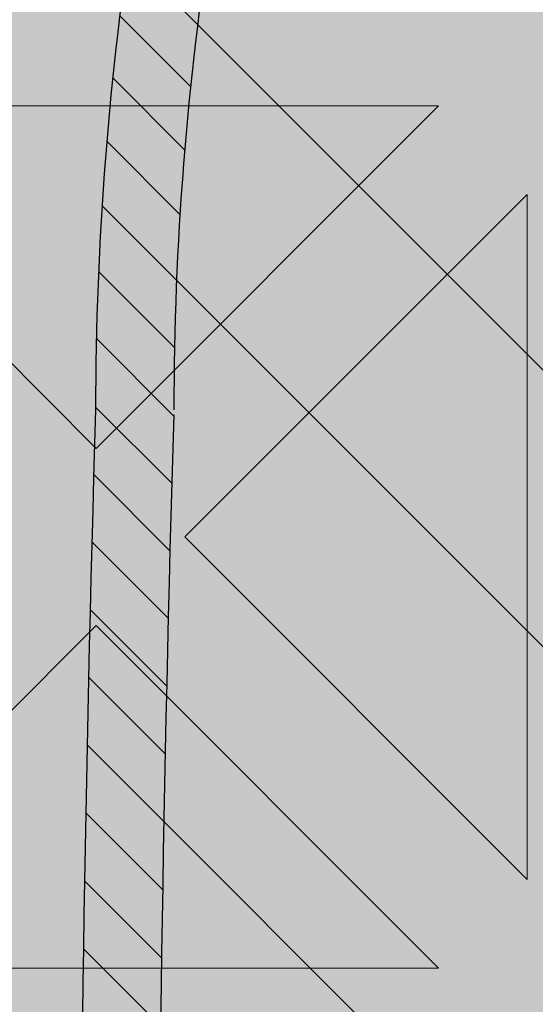
# Model space of a CAD drawing. Units: inches. Extents: x 844 to 2234, y 346 to 1084.
# Tile 78 of 93: x 2000.116 to 2001.166, y 704.51 to 706.514. Entities that reach past the tile are written whole.
import ezdxf

# ---------------------------------------------------------------- set-up
doc = ezdxf.new("R2010")
doc.units = ezdxf.units.IN
doc.header["$MEASUREMENT"] = 0
for name, color, linetype, lineweight in [('A-ANNO-DIMS', 2, 'Continuous', 18), ('furniture', 8, 'Continuous', 18), ('RA-AP-01$0$INT', 35, 'Continuous', 5)]:
    doc.layers.add(name, color=color, linetype=linetype, lineweight=lineweight)
doc.layers.add('RA-AP-01$0$FURN', color=3, linetype='Continuous')
doc.layers.add('RA-AP-01$0$WOOD', color=64, linetype='Continuous')
doc.styles.get("Standard").update_dxf_attribs({"font": 'arial.ttf'})
doc.dimstyles.get("Standard").update_dxf_attribs({"dimtxt": 6, "dimasz": 3, "dimexe": 0.18, "dimexo": 0.0625, "dimgap": 0.09, "dimtad": 0, "dimtih": 1, "dimtoh": 1, "dimdec": 1, "dimzin": 0, "dimdsep": 46, "dimlunit": 3, "dimtxsty": 'Standard', "dimblk": 'ARCHTICK', "dimcen": 0.09, "dimadec": 0, "dimazin": 0, "dimtfac": 1, "dimtdec": 1, "dimtofl": 0, "dimtmove": 0, "dimatfit": 3, "dimfxl": 1, "dimtolj": 1, "dimtzin": 0, "dimarcsym": 0})

# ---------------------------------------------------------------- blocks, each defined once
blk = doc.blocks.new('A$C18D01794')
at = {"layer": 'RA-AP-01$0$INT'}
h = blk.add_hatch(color=256, dxfattribs=at)
h.paths.add_polyline_path([(4.585917135068448, -7.856712009587804), (4.614201406330596, -7.856712009587056), (4.668846067270487, -7.802067348644738), (4.723490728212344, -7.856712009584164), (4.771774999457151, -7.856712009582887), (4.826419660396886, -7.80206734864072), (4.862780050090322, -7.838427738332541), (4.844495778842715, -7.856712009580965), (4.862780050090411, -7.856712009580482), (4.905206456960182, -7.814285602707865), (4.947632863832445, -7.856712009578238), (4.965917135079675, -7.856712009577755), (4.947632863831759, -7.838427738330656), (4.983993253523576, -7.802067348637219), (5.038637914464627, -7.856712009575829), (5.08692218571208, -7.856712009574554), (5.141566846649976, -7.802067348634224), (5.196211507589851, -7.856712009571666), (5.224495778822615, -7.856712009570916), (4.905206456953975, -7.537422687702283)])
h.paths.add_polyline_path([(4.895206456956031, -7.575706958950402), (4.895206456958921, -7.684996280828174), (4.840561796018589, -7.630351619890275)], flags=16)
h.paths.add_polyline_path([(4.915206456955638, -7.575706958949956), (4.969851117895509, -7.630351619887399), (4.915206456957609, -7.684996280827732)], flags=16)
h.paths.add_polyline_path([(4.826419660395175, -7.644493755514321), (4.881064321335613, -7.699138416452331), (4.771774999456703, -7.69913841645522)], flags=16)
h.paths.add_polyline_path([(4.983993253519558, -7.644493755510815), (5.038637914460456, -7.699138416449285), (4.929348592581548, -7.69913841645126)], flags=16)
h.paths.add_polyline_path([(4.881064321336025, -7.719138416452334), (4.826419660397532, -7.773783077393256), (4.771774999457062, -7.719138416455217)], flags=16)
h.paths.add_polyline_path([(4.929348592582019, -7.71913841645126), (5.038637914460982, -7.719138416449284), (4.983993253522945, -7.773783077389749)], flags=16)
h.paths.add_polyline_path([(4.895206456960191, -7.733280552075633), (4.895206456962115, -7.806001331460164), (4.876922185715016, -7.824285602708492), (4.840561796021581, -7.787925213016675)], flags=16)
h.paths.add_polyline_path([(4.915206456958487, -7.733280552075187), (4.969851117899527, -7.787925213013798), (4.933490728206909, -7.824285602708034), (4.9152064569598, -7.806001331461736)], flags=16)
h.paths.add_polyline_path([(4.757632863832376, -7.733280552079264), (4.812277524772842, -7.787925213017304), (4.757632863834348, -7.842569873958233)], flags=16)
h.paths.add_polyline_path([(4.737632863832376, -7.73328055207979), (4.737632863834348, -7.842569873958701), (4.682988202893906, -7.787925213020692)], flags=16)
h.paths.add_polyline_path([(5.05278005008503, -7.733280552072701), (5.052780050087917, -7.842569873951664), (4.998135389146995, -7.787925213013169)], flags=16)
h.paths.add_polyline_path([(5.072780050085024, -7.733280552072333), (5.127424711025931, -7.787925213010806), (5.072780050087916, -7.842569873951244)], flags=16)
h.paths.add_polyline_path([(4.935917135072783, -7.506712009583784), (5.255206456948811, -7.826001331459767), (5.255206456948932, -7.797717060211899), (5.200561796010279, -7.743072399273238), (5.255206456949403, -7.688427738334128), (5.25520645694961, -7.640143467086677), (5.200561796009787, -7.585498806146837), (5.236922185702417, -7.549138416454212), (5.255206456949919, -7.56742268770172), (5.255206456949998, -7.549138416454178), (5.212780050078687, -7.506712009583814), (5.25520645695036, -7.464285602712145), (5.255206456950438, -7.446001331464763), (5.236922185702424, -7.464285602712779), (5.200561796009796, -7.427925213020149), (5.255206456950753, -7.373280552079203), (5.25520645695096, -7.324996280834394), (5.200561796010322, -7.270351619893748), (5.255206456951428, -7.215706958952649), (5.255206456951547, -7.187422687705071)])
h.paths.add_polyline_path([(5.042988202883395, -7.42792521302065), (5.097632863823085, -7.373280552080975), (5.097632863822622, -7.482569873959883)], flags=16)
h.paths.add_polyline_path([(5.028846067259663, -7.442067348644384), (5.083490728198774, -7.496712009583504), (4.974201406321001, -7.496712009583035)], flags=16)
h.paths.add_polyline_path([(5.117632863823087, -7.37328055208089), (5.172277524762331, -7.42792521302015), (5.11763286382262, -7.482569873959851)], flags=16)
h.paths.add_polyline_path([(5.08349072819877, -7.516712009582191), (5.028846067259652, -7.571356670521302), (4.974201406320998, -7.516712009582638)], flags=16)
h.paths.add_polyline_path([(5.131774999446817, -7.35913841645716), (5.186419660386065, -7.413783077396415), (5.241064321325782, -7.359138416456712)], flags=17)
h.paths.add_polyline_path([(5.131774999446228, -7.496712009583703), (5.186419660386065, -7.442067348643883), (5.222780050079488, -7.478427738337313), (5.204495778832781, -7.496712009584014)], flags=16)
h.paths.add_polyline_path([(5.097632863822613, -7.530854145205813), (5.097632863823061, -7.640143467084723), (5.042988202883383, -7.585498806145032)], flags=16)
h.paths.add_polyline_path([(5.131774999446899, -7.339138416457162), (5.241064321325809, -7.339138416456712), (5.186419660386591, -7.284493755517479)], flags=17)
h.paths.add_polyline_path([(5.131774999446226, -7.516712009581999), (5.204495778830767, -7.516712009581702), (5.22278005007868, -7.534996280829206), (5.186419660386049, -7.571356670521828)], flags=16)
h.paths.add_polyline_path([(5.11763286382262, -7.530854145205852), (5.17227752476232, -7.585498806145562), (5.117632863823064, -7.64014346708481)], flags=16)
h.paths.add_polyline_path([(5.186419660386069, -7.599640941770585), (5.241064321325754, -7.654285602710281), (5.131774999446791, -7.654285602709814)], flags=16)
h.paths.add_polyline_path([(5.131774999446872, -7.674285602709813), (5.24106432132578, -7.674285602710282), (5.186419660386554, -7.728930263649504)], flags=16)
h.paths.add_polyline_path([(5.255206456951811, -7.126001331467467), (5.255206456951895, -7.106712009588038), (4.555206456956052, -7.106712009588038), (4.555206456956136, -7.12600133146746), (4.905206456953973, -7.476001331465289)])
h.paths.add_polyline_path([(4.983993253513404, -7.368930263651977), (4.92934859257295, -7.314285602713969), (5.03863791445186, -7.314285602711063)], flags=16)
h.paths.add_polyline_path([(4.969851117889988, -7.383072399276016), (4.915206456952556, -7.437717060215906), (4.915206456949648, -7.328427738338133)], flags=16)
h.paths.add_polyline_path([(4.929348592572535, -7.294285602713971), (4.983993253511019, -7.239640941773039), (5.038637914451496, -7.294285602711065)], flags=16)
h.paths.add_polyline_path([(5.052780050074912, -7.280143467087016), (4.998135389134438, -7.225498806148989), (5.052780050072919, -7.170854145208052)], flags=16)
h.paths.add_polyline_path([(5.07278005007491, -7.280143467086489), (5.072780050072918, -7.170854145207579), (5.127424711013374, -7.225498806145578)], flags=16)
h.paths.add_polyline_path([(4.89520645695295, -7.437717060216355), (4.840561796013067, -7.383072399278919), (4.895206456950961, -7.328427738338582)], flags=16)
h.paths.add_polyline_path([(4.915206456948365, -7.280143467090674), (4.915206456946434, -7.207422687704125), (4.933490728192729, -7.18913841645701), (4.969851117886972, -7.225498806149623)], flags=16)
h.paths.add_polyline_path([(4.881064321327021, -7.314285602715054), (4.82641966038902, -7.368930263655506), (4.771774999448108, -7.314285602717047)], flags=16)
h.paths.add_polyline_path([(4.895206456950073, -7.280143467091125), (4.840561796009022, -7.225498806152518), (4.876922185700835, -7.18913841645908), (4.895206456948749, -7.207422687706589)], flags=16)
h.paths.add_polyline_path([(4.983993253510392, -7.211356670525576), (4.947632863816944, -7.174996280833758), (4.965917135064043, -7.156712009585847), (5.038637914448995, -7.156712009584522)], flags=16)
h.paths.add_polyline_path([(4.881064321326543, -7.294285602715056), (4.771774999447578, -7.294285602717046), (4.826419660385607, -7.239640941776569)], flags=16)
h.paths.add_polyline_path([(4.905206456946447, -7.19913841645844), (4.862780050074785, -7.156712009587725), (4.947632863816685, -7.156712009586302)], flags=16)
h.paths.add_polyline_path([(5.14156684663679, -7.211356670521528), (5.086922185696452, -7.156712009583639), (5.196211507574223, -7.156712009581651)], flags=16)
h.paths.add_polyline_path([(4.8264196603837, -7.211356670529104), (4.771774999442643, -7.156712009590501), (4.8444957788276, -7.156712009588568), (4.862780050075511, -7.17499628083566)], flags=16)
h.paths.add_polyline_path([(4.812277524760289, -7.225498806153156), (4.757632863822258, -7.28014346709363), (4.757632863819352, -7.170854145214669)], flags=16)
h.paths.add_polyline_path([(4.73763286382226, -7.280143467093997), (4.682988202881349, -7.22549880615554), (4.737632863819352, -7.170854145215086)], flags=16)
h.paths.add_polyline_path([(4.723490728195188, -7.156712009591787), (4.668846067257299, -7.211356670532127), (4.614201406317417, -7.156712009594693)], flags=16)
h.paths.add_polyline_path([(4.597632863829262, -7.506712009583814), (4.555206456957951, -7.54913841645418), (4.555206456958029, -7.56742268770172), (4.573490728205535, -7.549138416454212), (4.609851117898167, -7.585498806146839), (4.555206456958338, -7.640143467086675), (4.555206456958546, -7.688427738334125), (4.60985111789767, -7.743072399273238), (4.555206456959015, -7.797717060211899), (4.555206456959138, -7.826001331459767), (4.874495778835167, -7.506712009583786), (4.5552064569564, -7.187422687705062), (4.555206456956523, -7.215706958952644), (4.609851117897629, -7.270351619893746), (4.555206456956988, -7.324996280834396), (4.555206456957198, -7.373280552079195), (4.609851117898153, -7.427925213020147), (4.573490728205528, -7.464285602712779), (4.555206456957507, -7.446001331464756), (4.555206456957585, -7.464285602712143)])
h.paths.add_polyline_path([(4.712780050085332, -7.482569873959882), (4.712780050084863, -7.373280552080972), (4.767424711024555, -7.42792521302065)], flags=16)
h.paths.add_polyline_path([(4.726922185709173, -7.496712009583504), (4.781566846648288, -7.442067348644384), (4.836211507586949, -7.496712009583033)], flags=16)
h.paths.add_polyline_path([(4.692780050085327, -7.482569873959851), (4.638135389145619, -7.427925213020149), (4.692780050084865, -7.373280552080892)], flags=16)
h.paths.add_polyline_path([(4.726922185709182, -7.516712009582191), (4.836211507586949, -7.51671200958264), (4.7815668466483, -7.571356670521304)], flags=16)
h.paths.add_polyline_path([(4.678637914461726, -7.496712009583706), (4.605917135075169, -7.496712009584014), (4.587632863828464, -7.478427738337311), (4.623993253521887, -7.442067348643881)], flags=16)
h.paths.add_polyline_path([(4.712780050085336, -7.530854145205816), (4.767424711024568, -7.585498806145034), (4.71278005008489, -7.640143467084724)], flags=16)
h.paths.add_polyline_path([(4.678637914461726, -7.516712009582001), (4.623993253521899, -7.571356670521829), (4.587632863829271, -7.534996280829206), (4.605917135077185, -7.5167120095817)], flags=16)
h.paths.add_polyline_path([(4.692780050085336, -7.530854145205848), (4.692780050084889, -7.64014346708481), (4.638135389145632, -7.585498806145562)], flags=16)
h.paths.add_polyline_path([(4.623993253521885, -7.413783077396415), (4.678637914461131, -7.359138416457161), (4.56934859258217, -7.359138416456712)], flags=17)
h.paths.add_polyline_path([(4.623993253521901, -7.599640941770568), (4.678637914461158, -7.654285602709814), (4.569348592582195, -7.654285602710281)], flags=16)
h.paths.add_polyline_path([(4.678637914461051, -7.339138416457162), (4.623993253521361, -7.284493755517479), (4.569348592582143, -7.339138416456712)], flags=17)
h.paths.add_polyline_path([(4.678637914461076, -7.674285602709813), (4.623993253521399, -7.728930263649504), (4.569348592582167, -7.674285602710281)], flags=16)
h = blk.add_hatch(color=256, dxfattribs=at)
h.paths.add_polyline_path([(5.028846067259997, -7.571356670520955), (4.974201406321342, -7.516712009582294), (5.083490728199115, -7.516712009581846)])
h.paths.add_polyline_path([(4.974201406321344, -7.496712009582688), (5.028846067260004, -7.442067348644037), (5.083490728199117, -7.496712009583157)])
h.paths.add_polyline_path([(5.042988202883738, -7.427925213020309), (5.097632863823428, -7.373280552080627), (5.097632863822963, -7.482569873959537)])
h.paths.add_polyline_path([(5.117632863822961, -7.482569873959509), (5.117632863823428, -7.373280552080546), (5.172277524762674, -7.427925213019804)])
h.paths.add_polyline_path([(5.131774999446572, -7.496712009583358), (5.186419660386406, -7.442067348643536), (5.222780050079831, -7.478427738336961), (5.204495778833122, -7.496712009583667)])
h.paths.add_polyline_path([(5.236922185702764, -7.464285602712433), (5.200561796010139, -7.427925213019802), (5.255206456949971, -7.373280552079975), (5.255206456950271, -7.446001331464927)])
h.paths.add_polyline_path([(5.186419660386412, -7.41378307739607), (5.131774999447164, -7.359138416456815), (5.241064321326123, -7.359138416456366)])
h.paths.add_polyline_path([(5.131774999447238, -7.339138416456815), (5.186419660386934, -7.284493755517132), (5.241064321326153, -7.339138416456368)])
h.paths.add_polyline_path([(5.200561796010663, -7.270351619893402), (5.255206456949324, -7.215706958954747), (5.255206456949777, -7.324996280832518)])
h.paths.add_polyline_path([(5.21278005007903, -7.50671200958347), (5.255206456950223, -7.464285602712278), (5.255206456950696, -7.549138416454185)])
h.paths.add_polyline_path([(5.13177499944657, -7.516712009581652), (5.204495778831106, -7.516712009581354), (5.222780050079024, -7.534996280828858), (5.186419660386397, -7.571356670521485)])
h.paths.add_polyline_path([(5.117632863823405, -7.640143467084465), (5.117632863822955, -7.530854145205498), (5.172277524762665, -7.585498806145217)])
h.paths.add_polyline_path([(5.042988202883727, -7.585498806144689), (5.097632863822957, -7.530854145205474), (5.097632863823407, -7.64014346708438)])
h.paths.add_polyline_path([(5.131774999447135, -7.654285602709467), (5.186419660386394, -7.599640941770219), (5.241064321326097, -7.654285602709933)])
h.paths.add_polyline_path([(5.200561796010128, -7.585498806146492), (5.236922185702758, -7.549138416453866), (5.255206456950264, -7.567422687701371), (5.255206456949948, -7.640143467086325)])
h.paths.add_polyline_path([(5.186419660386895, -7.728930263649157), (5.131774999447213, -7.674285602709467), (5.241064321326127, -7.674285602709934)])
h.paths.add_polyline_path([(5.200561796010624, -7.743072399272893), (5.255206456949745, -7.688427738333778), (5.255206456949276, -7.797717060211553)])
for p, q in [((5.131774999446817, -7.359138416457161), (5.24106432132578, -7.359138416456712)), ((5.131774999446817, -7.359138416457161), (5.186419660386065, -7.413783077396415)), ((5.24106432132578, -7.359138416456712), (5.186419660386065, -7.413783077396415)), ((5.117632863823085, -7.37328055208089), (5.172277524762331, -7.427925213020149)), ((5.117632863823085, -7.37328055208089), (5.11763286382262, -7.482569873959853)), ((5.11763286382262, -7.482569873959853), (5.172277524762331, -7.427925213020149)), ((5.131774999446229, -7.496712009583704), (5.186419660386063, -7.442067348643881)), ((5.186419660386062, -7.442067348643881), (5.222780050078687, -7.478427738336511)), ((5.204495778831181, -7.496712009584014), (5.131774999446229, -7.496712009583704))]:
    blk.add_line(p, q, dxfattribs=at)
blk = doc.blocks.new('A$C32926AE1')
at = {"layer": 'RA-AP-01$0$WOOD'}
h = blk.add_hatch(color=256, dxfattribs=at)
h.dxf.hatch_style = 1
h.paths.add_polyline_path([(5.157430609644524, 4.573483066760929, -0.1009492694046607), (5.155401577623758, 4.593365984175333, -0.1842662638101597), (5.172249623284174, 4.638795604568598, 0.2056608120311276), (5.179560981299304, 4.661316324430096, 0.3614336704623542), (5.134352340494423, 4.706524965234944, 0.2056608120311297), (5.111831620632933, 4.699213607219793, -0.1842662638101113), (5.066402000239693, 4.682365561559342, -0.1055311479399994), (5.045656153913092, 4.68467289944697, 0.1567636581983829), (4.763886414745334, 4.684672899446966, -0.1055311479399895), (4.743140568418733, 4.68236556155934, -0.1842662638100833), (4.6977109480255, 4.69921360721979, 0.2056608120302612), (4.675190228164109, 4.706524965234949, 0.3614336704708441), (4.629981587358889, 4.66131632442871, 0.2056608120245944), (4.637292945374126, 4.638795604567974, -0.1842662638101024), (4.654140991034615, 4.59336598417475, -0.1009492694055169), (4.652111959013835, 4.573483066760181, 0.021410119221476), (4.629748025606143, 4.156712009541676, 0.0214101192214795), (4.652111959013809, 3.739940952323101, -0.1009492694059586), (4.654140991034615, 3.720058034908448, -0.1842662638100975), (4.637292945374126, 3.674628414515226, 0.2056608120245705), (4.629981587358889, 3.652107694654492, 0.3614336704708879), (4.675190228164113, 3.606899053848249, 0.2056608120302384), (4.697710948025501, 3.614210411863408, -0.1842662638100995), (4.743140568418738, 3.63105845752386, -0.1055311479402541), (4.763886414745388, 3.628751119636215, 0.1567636581983776), (5.045656153913137, 3.628751119636244, -0.1055311479397538), (5.066402000239692, 3.631058457523857, -0.1842662638101067), (5.111831620632931, 3.614210411863407, 0.2056608120310924), (5.134352340494417, 3.606899053848256, 0.3614336704624001), (5.179560981299307, 3.652107694653103, 0.2056608120311314), (5.172249623284175, 3.6746284145146, -0.1842662638101402), (5.155401577623758, 3.72005803490786, -0.1009492694051366), (5.15743060964455, 3.739940952322354, 0.0214101192215073), (5.179794543052287, 4.156712009541468, 0.0214101192215252)])
h.paths.add_polyline_path([(4.639748609479751, 4.156712009541513, 0.0213537860821624), (4.661970494867118, 3.741887061152232, -0.094075836301374), (4.664143710413708, 3.7196126951003, -0.1824818158568985), (4.644813765429836, 3.668037719127816, 0.2056608120245319), (4.639939526753007, 3.653023905887301, 0.3614336704710246), (4.676106439397173, 3.616856993242342, 0.2056608120302234), (4.691120252638095, 3.621731231919122, -0.1824818158602558), (4.742695228611606, 3.641061176902986, -0.1029891339458722), (4.766991894714349, 3.638256818950944, 0.156709409989566), (5.042550673941472, 3.638256818950105, -0.102989133958497), (5.066847340047078, 3.641061176902949, -0.1824818158594995), (5.118422316020358, 3.621731231919103, 0.2056608120311416), (5.133436129261316, 3.616856993242346, 0.3614336704621468), (5.169603041905217, 3.653023905886178, 0.2056608120310986), (5.164728803228477, 3.668037719127177, -0.1824818158565612), (5.145398858244737, 3.719612695099578, -0.0940758363009313), (5.147572073791232, 3.741887061151398, 0.0213537860822023), (5.169793959178681, 4.156712009541451, 0.0213537860822226), (5.147572073791203, 4.571536957931898, -0.0940758363005034), (5.145398858244737, 4.59381132398362, -0.1824818158565587), (5.164728803228476, 4.645386299956021, 0.2056608120311045), (5.169603041905216, 4.66040011319702, 0.3614336704621845), (5.133436129261313, 4.696567025840856, 0.2056608120310773), (5.118422316020359, 4.691692787164098, -0.182481815859508), (5.066847340047078, 4.67236284218025, -0.1029891339584606), (5.04255067394148, 4.675167200133092, 0.156709409989566), (4.766991894714357, 4.675167200132257, -0.1029891339458842), (4.742695228611611, 4.672362842180213, -0.1824818158602725), (4.691120252638095, 4.691692787164077, 0.2056608120302152), (4.676106439397174, 4.696567025840858, 0.3614336704710363), (4.639939526753005, 4.660400113195899, 0.2056608120245495), (4.644813765429837, 4.645386299955384, -0.1824818158568934), (4.664143710413708, 4.593811323982902, -0.0940758363009187), (4.661970494867149, 4.571536957931074, 0.021353786082177)], flags=16)
h.paths.add_polyline_path([(5.129794543052235, 4.432167055276933, -0.0141661062790638), (5.130152669293814, 4.156927903047693, -0.0141661062790647), (5.129794543052234, 3.881688750818433, -0.0785247771143638), (5.10979738006795, 3.755143611847103, 0.0945969212073497), (5.105408519571111, 3.717898134952927, 0.1043170707844957), (5.116074640131521, 3.670385395016088, 0.1043170707864965), (5.068561900193738, 3.681051515576561, 0.09459692119553), (5.031316423304057, 3.676662655080835, -0.1580239521427272), (4.778226145355827, 3.676662655080367, 0.0945969211986668), (4.740980668464973, 3.681051515576592, 0.1043170707882822), (4.693467928526415, 3.670385395015844, 0.1043170707867916), (4.704134049087309, 3.717898134953662, 0.0945969211972894), (4.69974518859162, 3.755143611844042, -0.0785247771163196), (4.679748025606343, 3.881688750818406, -0.0141661062790663), (4.679389899364763, 4.156927903047693, -0.0141661062790672), (4.679748025606343, 4.432167055276998, -0.0785247771163064), (4.699745188591625, 4.55871219425134, 0.094596921197333), (4.704134049087308, 4.595957671141738, 0.1043170707867205), (4.693467928526416, 4.643470411079523, 0.1043170707882628), (4.740980668464965, 4.632804290518776, 0.0945969211988114), (4.778226145355874, 4.637193151015016, -0.158023952142669), (5.031316423304015, 4.637193151014546, 0.0945969211956361), (5.068561900193736, 4.632804290518806, 0.1043170707864979), (5.11607464013152, 4.643470411079278, 0.1043170707844617), (5.105408519571112, 4.595957671142455, 0.0945969212074597), (5.109797380067959, 4.558712194248236, -0.0785247771143467)], flags=0)
h.paths.add_polyline_path([(5.119794532311105, 4.432259799204851, -0.0142000800617244), (5.120156169157484, 4.156927903047701, -0.0142000800617277), (5.119794532311105, 3.881596006890482, -0.0784894509520253), (5.100273383573699, 3.758192358677797, 0.0940138827242913), (5.095413455884425, 3.717477693979438, 0.0606271852308753), (5.099615656341024, 3.686844378806616, 0.0606271852322524), (5.068982341167493, 3.691046579263239, 0.0940138827010453), (5.028267676478798, 3.686186651576848, -0.1580706864508061), (4.781274892180912, 3.686186651576435, 0.0940138827026903), (4.740560227491556, 3.691046579263279, 0.0606271852339895), (4.709926912317155, 3.686844378806508, 0.0606271852329405), (4.714129112773991, 3.717477693980356, 0.094013882701304), (4.709269185087677, 3.758192358669163, -0.0784894509577193), (4.689748036347473, 3.881596006890469, -0.014200080061729), (4.689386399501094, 4.156927903047709, -0.0142000800617217), (4.689748036347473, 4.432259799204808, -0.078489450957724), (4.709269185087651, 4.555663447426125, 0.0940138827014585), (4.714129112773992, 4.596378112114996, 0.0606271852329731), (4.709926912317154, 4.62701142728886, 0.0606271852340196), (4.74056022749157, 4.622809226832087, 0.0940138827024997), (4.781274892180847, 4.627669154518912, -0.1580706864508359), (5.028267676478777, 4.627669154518526, 0.0940138827010946), (5.068982341167492, 4.622809226832129, 0.060627185232254), (5.099615656341024, 4.627011427288751, 0.0606271852308727), (5.095413455884425, 4.59637811211593, 0.0940138827241088), (5.100273383573675, 4.555663447417647, -0.0784894509520978)], flags=0)
h.paths.add_polyline_path([(5.06978912287499, 4.430218106756144, -0.014241683694547), (5.070173729147532, 4.156927903047672, -0.0142416836945458), (5.06978912287499, 3.883637699339223, -0.0800609523125196), (5.052662118612511, 3.773463122773442, 0.0526421978001116), (5.04590916754064, 3.740550867606997, 0.0526421977992423), (5.012996912374707, 3.73379791653534, -0.1583028414718258), (4.796545656286308, 3.73379791653451, 0.0526421978034211), (4.763633401117837, 3.740550867607021, 0.0526421978018622), (4.756880450045755, 3.773463122774558, -0.0800609523117106), (4.739753445783639, 3.883637699339268, -0.0142416836945435), (4.739368839511098, 4.156927903047671, -0.0142416836945477), (4.739753445783639, 4.430218106756155, -0.0800609523116345), (4.75688045004574, 4.540392683320762, 0.052642197801941), (4.763633401117837, 4.573304938488346, 0.0526421978035071), (4.796545656286361, 4.580057889560873, -0.1583028414717561), (5.012996912374669, 4.580057889560039, 0.0526421977993048), (5.04590916754064, 4.57330493848837, 0.0526421978002057), (5.052662118612529, 4.540392683321868, -0.080060952312477)], flags=0)
h.paths.add_polyline_path([(5.049789715110557, 4.43038092723357, -0.0143097550741839), (5.05018085590259, 4.156927903047715, -0.0143097550741854), (5.049789715110558, 3.883474878861827, -0.0800685599149176), (5.03362098255317, 3.779581877367999, 0.0306258898956367), (5.028241146483733, 3.758218888663947, 0.0306258898977031), (5.006878157778253, 3.75283905259408, -0.1583983521624096), (4.802664410878162, 3.752839052594731, 0.0306258898946014), (4.781301422174808, 3.758218888663924, 0.0306258898967912), (4.775921586105202, 3.779581877368794, -0.080068559914251), (4.759752853548071, 3.883474878861786, -0.0143097550741854), (4.759361712756037, 4.156927903047671, -0.0143097550741854), (4.759752853548071, 4.430380927233557, -0.0800685599142479), (4.775921586105193, 4.534273928726546, 0.0306258898968306), (4.781301422174808, 4.555636917431444, 0.0306258898945754), (4.802664410878143, 4.561016753500631, -0.1583983521624168), (5.006878157778244, 4.561016753501291, 0.0306258898977177), (5.028241146483733, 4.555636917431421, 0.0306258898958182), (5.03362098255321, 4.534273928727244, -0.080068559914796)], flags=0)
h.paths.add_polyline_path([(4.999766070382627, 4.428171244713864, -0.0143443147609634), (5.000198441819402, 4.156927903047689, -0.0143443147609612), (4.999766070382627, 3.885684561381556, -0.0784641635803329), (4.987356730658798, 3.799103304488872, -0.1506053783831347), (4.822185837999821, 3.79910330448882, -0.0784641635803318), (4.809776498276007, 3.885684561381509, -0.014344314760963), (4.809344126839227, 4.156927903047677, -0.0143443147609645), (4.809776498276007, 4.428171244713873, -0.0784641635803192), (4.822185837999822, 4.514752501606549, -0.1506053783831338), (4.987356730658798, 4.514752501606494, -0.078464163580285)], flags=0)
h.paths.add_polyline_path([(4.979755254238824, 4.42764379880488, -0.0143772539198268), (4.980205517789977, 4.156927903047693, -0.0143772539198275), (4.979755254238824, 3.886212007290489, -0.0689242507424422), (4.971183264704897, 3.815276770442801, -0.1296645318904179), (4.838359303953726, 3.815276770442746, -0.0689242507424186), (4.829787314419809, 3.886212007290419, -0.0143772539198292), (4.829337050868653, 4.156927903047653, -0.0143772539198325), (4.829787314419809, 4.427643798804946, -0.0689242507424211), (4.838359303953725, 4.498579035652621, -0.1296645318904187), (4.971183264704897, 4.498579035652565, -0.0689242507424401)], flags=0)
h = blk.add_hatch(color=256, dxfattribs=at)
h.dxf.hatch_style = 1
h.paths.add_polyline_path([(5.145398858244737, 4.59381132398362, -0.1824818158565616), (5.164728803228476, 4.645386299956021, 0.2056608120311045), (5.169603041905216, 4.66040011319702, 0.3614336704621845), (5.133436129261313, 4.696567025840856, 0.2056608120310773), (5.118422316020359, 4.691692787164098, -0.182481815859508), (5.066847340047078, 4.67236284218025, -0.1029891339584606), (5.04255067394148, 4.675167200133092, 0.156709409989566), (4.766991894714357, 4.675167200132257, -0.1029891339458842), (4.742695228611611, 4.672362842180213, -0.1824818158602725), (4.691120252638095, 4.691692787164077, 0.2056608120302152), (4.676106439397174, 4.696567025840858, 0.3614336704710363), (4.639939526753005, 4.660400113195899, 0.2056608120245495), (4.644813765429837, 4.645386299955384, -0.1824818158568934), (4.664143710413708, 4.593811323982902, -0.0940758363009187), (4.661970494867149, 4.571536957931074, 0.0213537860821772), (4.639748609479751, 4.156712009541507, 0.0213537860821625), (4.661970494867119, 3.741887061152226, -0.0940758363013071), (4.664143710413708, 3.719612695100309, -0.1824818158569294), (4.644813765429836, 3.668037719127816, 0.2056608120245319), (4.639939526753007, 3.653023905887301, 0.3614336704710246), (4.676106439397173, 3.616856993242342, 0.2056608120302234), (4.691120252638095, 3.621731231919122, -0.1824818158602558), (4.742695228611606, 3.641061176902986, -0.1029891339458722), (4.766991894714349, 3.638256818950944, 0.156709409989566), (5.042550673941472, 3.638256818950105, -0.102989133958497), (5.066847340047078, 3.641061176902949, -0.1824818158594995), (5.118422316020358, 3.621731231919103, 0.2056608120311416), (5.133436129261316, 3.616856993242346, 0.3614336704621468), (5.169603041905217, 3.653023905886178, 0.2056608120310986), (5.164728803228477, 3.668037719127177, -0.1824818158565612), (5.145398858244737, 3.719612695099578, -0.0940758363009313), (5.147572073791232, 3.741887061151398, 0.0213537860822023), (5.169793959178681, 4.156712009541451, 0.0213537860822226), (5.147572073791203, 4.571536957931898, -0.0940758363004996)])
h.paths.add_polyline_path([(5.109797380067958, 4.55871219424824, -0.0785247771143472), (5.129794543052234, 4.432167055276936, -0.0141661062790644), (5.130152669293814, 4.156927903047685, -0.014166106279066), (5.129794543052234, 3.881688750818401, -0.0785247771143517), (5.109797380067946, 3.755143611847092, 0.0945969212073132), (5.105408519571111, 3.717898134952929, 0.1043170707844995), (5.116074640131521, 3.670385395016088, 0.1043170707864965), (5.068561900193738, 3.681051515576561, 0.09459692119553), (5.031316423304057, 3.676662655080835, -0.1580239521427272), (4.778226145355827, 3.676662655080367, 0.0945969211986668), (4.740980668464973, 3.681051515576592, 0.1043170707882822), (4.693467928526415, 3.670385395015844, 0.1043170707867916), (4.704134049087309, 3.717898134953662, 0.0945969211972894), (4.69974518859162, 3.755143611844042, -0.0785247771163196), (4.679748025606343, 3.881688750818406, -0.0141661062790663), (4.679389899364763, 4.156927903047693, -0.0141661062790672), (4.679748025606343, 4.432167055276998, -0.0785247771163064), (4.699745188591625, 4.55871219425134, 0.094596921197333), (4.704134049087308, 4.595957671141738, 0.1043170707867205), (4.693467928526416, 4.643470411079523, 0.1043170707882628), (4.740980668464965, 4.632804290518776, 0.0945969211988114), (4.778226145355874, 4.637193151015016, -0.158023952142669), (5.031316423304015, 4.637193151014546, 0.0945969211956361), (5.068561900193736, 4.632804290518806, 0.1043170707864979), (5.11607464013152, 4.643470411079278, 0.1043170707844617), (5.105408519571112, 4.595957671142455, 0.0945969212074504)], flags=16)
h.paths.add_polyline_path([(5.100273383573655, 4.55566344741771, -0.0784894509521388), (5.119794532311105, 4.432259799204852, -0.0142000800617252), (5.120156169157484, 4.156927903047686, -0.014200080061726), (5.119794532311105, 3.881596006890502, -0.0784894509520446), (5.100273383573696, 3.758192358677786, 0.0940138827242721), (5.095413455884425, 3.717477693979436, 0.0606271852308692), (5.099615656341024, 3.686844378806616, 0.0606271852322522), (5.068982341167493, 3.691046579263239, 0.0940138827010453), (5.028267676478798, 3.686186651576848, -0.1580706864508061), (4.781274892180912, 3.686186651576435, 0.0940138827026903), (4.740560227491556, 3.691046579263279, 0.0606271852339895), (4.709926912317155, 3.686844378806508, 0.0606271852329405), (4.714129112773991, 3.717477693980356, 0.094013882701304), (4.709269185087677, 3.758192358669163, -0.0784894509577193), (4.689748036347473, 3.881596006890469, -0.014200080061729), (4.689386399501094, 4.156927903047709, -0.0142000800617217), (4.689748036347473, 4.432259799204808, -0.078489450957724), (4.709269185087651, 4.555663447426125, 0.0940138827014585), (4.714129112773992, 4.596378112114996, 0.0606271852329731), (4.709926912317154, 4.62701142728886, 0.0606271852340196), (4.74056022749157, 4.622809226832087, 0.0940138827024997), (4.781274892180847, 4.627669154518912, -0.1580706864508359), (5.028267676478777, 4.627669154518526, 0.0940138827010946), (5.068982341167492, 4.622809226832129, 0.060627185232254), (5.099615656341024, 4.627011427288751, 0.0606271852308727), (5.095413455884425, 4.59637811211593, 0.094013882723957)], flags=0)
h.paths.add_polyline_path([(5.04590916754064, 4.57330493848837, 0.0526421978002057), (5.052662118612529, 4.540392683321868, -0.0800609523124783), (5.06978912287499, 4.430218106756142, -0.0142416836945469), (5.070173729147532, 4.156927903047672, -0.0142416836945458), (5.06978912287499, 3.883637699339223, -0.0800609523125196), (5.052662118612511, 3.773463122773442, 0.0526421978001116), (5.04590916754064, 3.740550867606997, 0.0526421977992423), (5.012996912374707, 3.73379791653534, -0.1583028414718258), (4.796545656286308, 3.73379791653451, 0.0526421978034211), (4.763633401117837, 3.740550867607021, 0.0526421978018622), (4.756880450045755, 3.773463122774558, -0.0800609523117106), (4.739753445783639, 3.883637699339268, -0.0142416836945435), (4.739368839511098, 4.156927903047671, -0.0142416836945477), (4.739753445783639, 4.430218106756155, -0.0800609523116345), (4.75688045004574, 4.540392683320762, 0.052642197801941), (4.763633401117837, 4.573304938488346, 0.0526421978035071), (4.796545656286361, 4.580057889560873, -0.1583028414717561), (5.012996912374669, 4.580057889560039, 0.0526421977993048)], flags=0)
h.paths.add_polyline_path([(5.028241146483733, 4.555636917431422, 0.0306258898956949), (5.033620982553182, 4.534273928727329, -0.0800685599148649), (5.049789715110557, 4.430380927233569, -0.0143097550741839), (5.05018085590259, 4.156927903047715, -0.0143097550741854), (5.049789715110558, 3.883474878861827, -0.0800685599149176), (5.03362098255317, 3.779581877367999, 0.0306258898956367), (5.028241146483733, 3.758218888663947, 0.0306258898977031), (5.006878157778253, 3.75283905259408, -0.1583983521624096), (4.802664410878162, 3.752839052594731, 0.0306258898946014), (4.781301422174808, 3.758218888663924, 0.0306258898967912), (4.775921586105202, 3.779581877368794, -0.080068559914251), (4.759752853548071, 3.883474878861786, -0.0143097550741854), (4.759361712756037, 4.156927903047671, -0.0143097550741854), (4.759752853548071, 4.430380927233557, -0.0800685599142479), (4.775921586105193, 4.534273928726546, 0.0306258898968306), (4.781301422174808, 4.555636917431444, 0.0306258898945754), (4.802664410878143, 4.561016753500631, -0.1583983521624168), (5.006878157778244, 4.561016753501291, 0.0306258898977174)], flags=0)
h.paths.add_polyline_path([(4.987356730658798, 4.514752501606494, -0.0784641635803018), (4.999766070382627, 4.428171244713845, -0.0143443147609637), (5.000198441819402, 4.156927903047665, -0.0143443147609622), (4.999766070382628, 3.885684561381514, -0.0784641635802952), (4.987356730658797, 3.799103304488872, -0.1506053783831338), (4.822185837999821, 3.799103304488819, -0.0784641635803342), (4.809776498276007, 3.885684561381512, -0.0143443147609628), (4.809344126839227, 4.156927903047676, -0.0143443147609646), (4.809776498276007, 4.428171244713873, -0.0784641635803192), (4.822185837999822, 4.514752501606549, -0.1506053783831338)], flags=0)
h.paths.add_polyline_path([(4.971183264704897, 4.498579035652566, -0.0689242507424384), (4.979755254238824, 4.427643798804883, -0.0143772539198276), (4.980205517789977, 4.15692790304768, -0.0143772539198258), (4.979755254238823, 3.88621200729051, -0.0689242507424628), (4.971183264704897, 3.815276770442801, -0.129664531890417), (4.838359303953726, 3.815276770442746, -0.0689242507424186), (4.829787314419809, 3.886212007290419, -0.0143772539198292), (4.829337050868653, 4.156927903047653, -0.0143772539198325), (4.829787314419809, 4.427643798804946, -0.0689242507424211), (4.838359303953725, 4.498579035652621, -0.1296645318904187)], flags=0)
h = blk.add_hatch(dxfattribs=at)
h.set_pattern_fill('ANSI31', color=256, scale=0.05, style=0)
h.set_pattern_definition([(45, (0, 0), (-0.0044194173824159, 0.0044194173824159), [])])
h.paths.add_polyline_path([(5.130152669293814, 4.156927903047704, 0.0141661062790657), (5.129794543052234, 4.432167055276982, 0.0777827904001433), (5.110168979996553, 4.557559993161921, -0.0976515123401879), (5.105408519571111, 4.595957671142454, -0.1043170707844687), (5.116074640131522, 4.64347041107928), (5.099615656341024, 4.627011427288751, 0.0606271852308727), (5.095413455884425, 4.59637811211593, 0.0940138827241088), (5.100273383573675, 4.555663447417647, -0.0784894509520972), (5.119794532311105, 4.432259799204852, -0.0142000800617252), (5.120156169157484, 4.156927903047686, -0.014200080061726), (5.119794532311105, 3.881596006890502, -0.0784894509520446), (5.100273383573696, 3.758192358677786, 0.0940138827242721), (5.095413455884425, 3.717477693979436, 0.0606271852308692), (5.099615656341024, 3.686844378806616), (5.116074640131519, 3.67038539501609, -0.1043170707844594), (5.105408519571112, 3.717898134952912, -0.0976515123401594), (5.11016897999655, 3.756295812933435, 0.0777827904001654), (5.129794543052234, 3.881688750818409, 0.0141661062790665)])
h.paths.add_polyline_path([(5.030164222210597, 3.676291055149937, -0.0976515123472002), (5.068561900193739, 3.681051515576561, -0.1043170707864927), (5.116074640131521, 3.670385395016088), (5.099615656341024, 3.686844378806616, 0.0606271852322522), (5.068982341167493, 3.691046579263239, 0.0940138827010453), (5.028267676478798, 3.686186651576848, -0.1580706864508061), (4.781274892180912, 3.686186651576435, 0.0940138827026903), (4.740560227491556, 3.691046579263279, 0.0606271852339913), (4.709926912317154, 3.686844378806508), (4.693467928526416, 3.670385395015845, -0.1043170707882796), (4.740980668464973, 3.681051515576592, -0.0976515123427246), (4.779378346446416, 3.676291055150394, 0.156512506893803)])
h.paths.add_polyline_path([(4.689748036347473, 3.881596006890472, -0.014200080061729), (4.689386399501094, 4.156927903047712, -0.0142000800617195), (4.689748036347473, 4.432259799204768, -0.078489450957742), (4.709269185087648, 4.555663447426114, 0.0940138827014821), (4.714129112773992, 4.596378112114995, 0.0606271852329748), (4.709926912317154, 4.62701142728886), (4.693467928526414, 4.643470411079524, -0.1043170707867939), (4.704134049087309, 4.595957671141706, -0.09765151234893), (4.699373588660725, 4.557559993157876, 0.0777827903975372), (4.679748025606343, 4.432167055276987, 0.0141661062790675), (4.679389899364763, 4.156927903047675, 0.0141661062790641), (4.679748025606343, 3.88168875081843, 0.0777827903975637), (4.699373588660724, 3.756295812937497, -0.0976515123490278), (4.704134049087308, 3.717898134953629, -0.1043170707867196), (4.693467928526416, 3.670385395015845), (4.709926912317155, 3.686844378806508, 0.0606271852329413), (4.714129112773991, 3.717477693980357, 0.0940138827013084), (4.709269185087676, 3.758192358669166, -0.0784894509577192)])
h.paths.add_polyline_path([(4.779378346446434, 4.63756475094498, -0.0976515123427943), (4.740980668464964, 4.632804290518776, -0.1043170707882609), (4.693467928526416, 4.643470411079523), (4.709926912317154, 4.62701142728886, 0.0606271852340196), (4.74056022749157, 4.622809226832087, 0.0940138827024997), (4.781274892180847, 4.627669154518912, -0.1580706864508359), (5.028267676478777, 4.627669154518526, 0.0940138827010946), (5.068982341167492, 4.622809226832129, 0.060627185232254), (5.099615656341024, 4.627011427288751), (5.116074640131521, 4.643470411079279, -0.1043170707865022), (5.068561900193735, 4.632804290518806, -0.0976515123475899), (5.030164222210446, 4.637564750945479, 0.1565125068936924)])
h = blk.add_hatch(dxfattribs=at)
h.set_pattern_fill('ANSI32', color=256, scale=0.2, style=0)
h.set_pattern_definition([(45, (0, 0), (-0.0530330085889911, 0.0530330085889911), []), (45, (0.035355339, 0), (-0.0530330085889911, 0.0530330085889911), [])])
h.paths.add_polyline_path([(5.119794532311105, 4.432259799204823, 0.0777015974868765), (5.10065834347252, 4.554469821747928, -0.0968902511992216), (5.095413455884425, 4.596378112115931, -0.060627185230871), (5.099615656341024, 4.627011427288751, -0.060627185232254), (5.068982341167492, 4.622809226832129, -0.0968902512198245), (5.027074050790956, 4.628054114423209, 0.1564657949319105), (4.782468517866163, 4.628054114422785, -0.0968902512152247), (4.740560227491555, 4.622809226832088, -0.0606271852339878), (4.709926912317155, 4.627011427288859, -0.0606271852329413), (4.714129112773991, 4.596378112115011, -0.0968902512205338), (4.708884225182929, 4.554469821738175, 0.0777015974804443), (4.689748036347473, 4.43225979920482, 0.0142000800617215), (4.689386399501094, 4.156927903047726, 0.0142000800617273), (4.689748036347473, 3.88159600689052, 0.077701597480541), (4.708884225182985, 3.759385984357019, -0.096890251220082), (4.714129112773992, 3.717477693980371, -0.0606271852329731), (4.709926912317154, 3.686844378806507, -0.060627185233988), (4.740560227491554, 3.691046579263279, -0.0968902512152569), (4.782468517866175, 3.685801691672578, 0.1564657949319236), (5.027074050790988, 3.685801691672169, -0.0968902512197451), (5.068982341167491, 3.691046579263239, -0.0606271852322557), (5.099615656341024, 3.686844378806616, -0.0606271852308727), (5.095413455884425, 3.717477693979438, -0.0968902511991229), (5.100658343472507, 3.7593859843474, 0.0777015974868745), (5.119794532311105, 3.8815960068905, 0.014200080061726), (5.120156169157484, 4.156927903047685, 0.0142000800617238)])
h.paths.add_polyline_path([(5.070173729147531, 4.156927903047684, -0.0142416836945481), (5.06978912287499, 3.883637699339191, -0.0800609523125107), (5.052662118612505, 3.773463122773424, 0.0526421978000811), (5.04590916754064, 3.740550867606997, 0.0526421977993214), (5.012996912374658, 3.733797916535325, -0.1583028414717916), (4.796545656286304, 3.733797916534512, 0.0526421978034138), (4.763633401117837, 3.740550867607021, 0.0526421978018622), (4.756880450045755, 3.773463122774558, -0.0800609523117106), (4.739753445783639, 3.883637699339268, -0.0142416836945435), (4.739368839511098, 4.156927903047671, -0.0142416836945477), (4.739753445783639, 4.430218106756155, -0.0800609523116345), (4.75688045004574, 4.540392683320762, 0.052642197801941), (4.763633401117837, 4.573304938488346, 0.0526421978035071), (4.796545656286361, 4.580057889560873, -0.1583028414717561), (5.012996912374669, 4.580057889560039, 0.0526421977993048), (5.04590916754064, 4.57330493848837, 0.0526421978002057), (5.052662118612529, 4.540392683321868, -0.0800609523124783), (5.06978912287499, 4.430218106756142, -0.0142416836945463)], flags=16)
h.paths.add_polyline_path([(5.050180855902591, 4.156927903047686, -0.0143097550741856), (5.049789715110558, 3.883474878861795, -0.0800685599148126), (5.033620982553202, 3.7795818773681, 0.0306258898957837), (5.028241146483733, 3.758218888663947, 0.0306258898977031), (5.006878157778253, 3.75283905259408, -0.1583983521624096), (4.802664410878162, 3.752839052594731, 0.0306258898946014), (4.781301422174808, 3.758218888663924, 0.0306258898967912), (4.775921586105202, 3.779581877368794, -0.080068559914251), (4.759752853548071, 3.883474878861786, -0.0143097550741854), (4.759361712756037, 4.156927903047671, -0.0143097550741854), (4.759752853548071, 4.430380927233557, -0.0800685599142479), (4.775921586105193, 4.534273928726546, 0.0306258898968306), (4.781301422174808, 4.555636917431444, 0.0306258898945754), (4.802664410878143, 4.561016753500631, -0.1583983521624168), (5.006878157778244, 4.561016753501291, 0.0306258898977177), (5.028241146483733, 4.555636917431421, 0.0306258898958182), (5.03362098255321, 4.534273928727244, -0.0800685599147973), (5.049789715110557, 4.430380927233568, -0.0143097550741854)], flags=0)
h.paths.add_polyline_path([(5.000198441819402, 4.15692790304769, -0.0143443147609622), (4.999766070382627, 3.885684561381539, -0.0784641635803169), (4.987356730658798, 3.799103304488873, -0.1506053783831347), (4.822185837999821, 3.79910330448882, -0.0784641635803318), (4.809776498276007, 3.885684561381509, -0.014344314760963), (4.809344126839227, 4.156927903047677, -0.0143443147609645), (4.809776498276007, 4.428171244713873, -0.0784641635803192), (4.822185837999822, 4.514752501606549, -0.1506053783831338), (4.987356730658798, 4.514752501606494, -0.0784641635803018), (4.999766070382627, 4.428171244713845, -0.0143443147609624)], flags=0)
h.paths.add_polyline_path([(4.980205517789976, 4.156927903047707, -0.0143772539198295), (4.979755254238824, 3.886212007290466, -0.06892425074242), (4.971183264704897, 3.815276770442801, -0.129664531890417), (4.838359303953726, 3.815276770442746, -0.0689242507424186), (4.829787314419809, 3.886212007290419, -0.0143772539198292), (4.829337050868653, 4.156927903047653, -0.0143772539198325), (4.829787314419809, 4.427643798804946, -0.0689242507424211), (4.838359303953725, 4.498579035652621, -0.1296645318904187), (4.971183264704897, 4.498579035652565, -0.0689242507424418), (4.979755254238824, 4.427643798804878, -0.0143772539198259)], flags=0)
for centre, radius, start, end in [((4.719397359771062, 4.432167055276791), 0.4103971832811724, 2.64254e-11, 17.95969975512227), ((4.719397359771062, 4.432167055276791), 0.4003971832811724, 2.64254e-11, 17.95969975512227), ((0.2735947217851873, 4.288228622620772), 4.858332530454211, 358.4526160002363, 1.697757744190978), ((0.2735875766687563, 4.288228324954387), 4.848346823659694, 358.4481555949444, 1.693297660527682)]:
    blk.add_arc(centre, radius, start, end, dxfattribs=at)
blk = doc.blocks.new('A$C5D2F253E')
at = {"layer": 'RA-AP-01$0$FURN', "xscale": -0.7999999999883585, "yscale": 0.7999999999883585, "zscale": 0.8, "rotation": 90}
blk.add_blockref('A$C18D01794', (-5.687757199772477, 4.75791982714071), dxfattribs=at)
at = {"layer": 'RA-AP-01$0$WOOD', "rotation": 270}
blk.add_blockref('A$C32926AE1', (-4.161339601644158, 5.73852594588169), dxfattribs=at)
blk = doc.blocks.new('_ArchTick')
at = {"color": 0, "linetype": 'ByBlock', "const_width": 0.15}
blk.add_lwpolyline([(-0.5, -0.5), (0.5, 0.5)], dxfattribs=at)
blk = doc.blocks.new('*D121')
at = {"layer": 'A-ANNO-DIMS', "color": 0, "lineweight": -2, "transparency": 16777216}
for p, q in [((2030.271987351997, 734.262611118704), (2040.245275089302, 734.262611118704)), ((2040.065275089302, 734.262611118704), (2040.065275089302, 704.6043509484256)), ((2040.065275089302, 668.557359536674), (2040.065275089302, 698.2156197069523)), ((2030.271987351997, 668.557359536674), (2040.245275089302, 668.557359536674))]:
    blk.add_line(p, q, dxfattribs=at)
at = {"layer": 'Defpoints', "color": 0, "transparency": 16777216}
for p in [(2030.209487351997, 734.262611118704), (2040.065275089302, 734.262611118704), (2030.209487351997, 668.557359536674)]:
    blk.add_point(p, dxfattribs=at)
at = {"layer": 'A-ANNO-DIMS', "color": 0, "lineweight": -2, "transparency": 16777216, "xscale": 3, "yscale": 3, "zscale": 3}
for p, rotation in [((2040.065275089302, 734.262611118704), 90), ((2040.065275089302, 668.557359536674), 270)]:
    blk.add_blockref('_ArchTick', p, dxfattribs=dict(at, rotation=rotation))
at = {"layer": 'A-ANNO-DIMS', "color": 0, "transparency": 16777216, "insert": (2040.065275089302, 701.4099853276883), "char_height": 6, "attachment_point": 5}
blk.add_mtext('\\A1;LOUNGE SET 5\'-5 1/2" TYP.', dxfattribs=at)

msp = doc.modelspace()

# ---------------------------------------------------------------- block references
at = {"layer": 'furniture', "xscale": -15.94108302203742, "yscale": 15.94108302203742, "zscale": 15.94108302203742, "rotation": 270}
msp.add_blockref('A$C5D2F253E', (1990.567271852805, 701.4028671565849), dxfattribs=at)

# ---------------------------------------------------------------- dimensions: what is measured, and where the dimension line sits
at = {"layer": 'A-ANNO-DIMS'}
dim = msp.add_linear_dim(base=(2040.065275089302, 734.262611118704), p1=(2030.209487351996, 668.5573595366737), p2=(2030.209487351996, 734.2626111187037), angle=90, text='LOUNGE SET <> TYP.', dimstyle='Standard', override={"dimdec": 1, "dimlfac": 1, "dimrnd": 0, "dimzin": 1, "dimdsep": 46, "dimlunit": 4, "dimfrac": 2}, dxfattribs=at)
dim.commit()
dim.dimension.update_dxf_attribs({"geometry": '*D121', "text_midpoint": (2040.065275089302, 701.4099853276883)})

doc.saveas('drawing.dxf')
